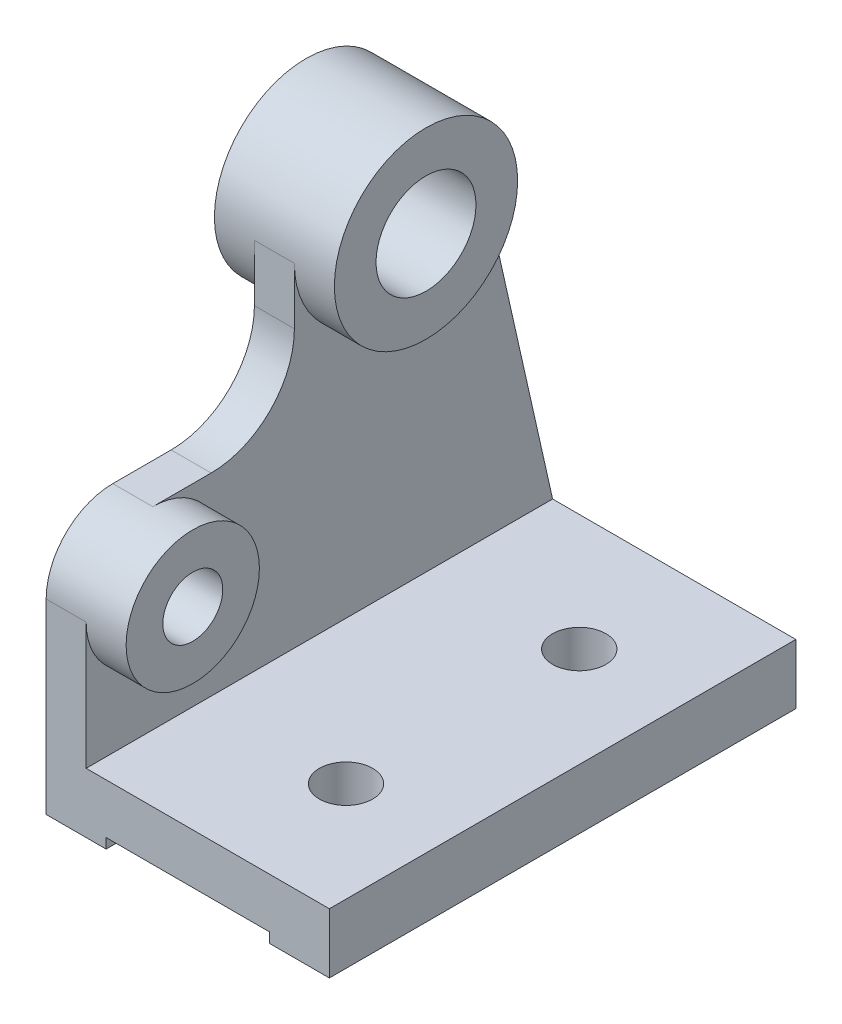
ISO-10303-21;
HEADER;
FILE_DESCRIPTION(('STEP AP214'),'2;1');
FILE_NAME('part.step','',(''),(''),'','','');
FILE_SCHEMA(('AUTOMOTIVE_DESIGN { 1 0 10303 214 1 1 1 1 }'));
ENDSEC;
DATA;
#1=APPLICATION_CONTEXT('core data for automotive mechanical design processes');
#2=APPLICATION_PROTOCOL_DEFINITION('international standard','automotive_design',2000,#1);
#3=PRODUCT_CONTEXT('',#1,'mechanical');
#4=PRODUCT('Part','Part','',(#3));
#5=PRODUCT_RELATED_PRODUCT_CATEGORY('part','',(#4));
#6=PRODUCT_DEFINITION_FORMATION('','',#4);
#7=PRODUCT_DEFINITION_CONTEXT('part definition',#1,'design');
#8=PRODUCT_DEFINITION('design','',#6,#7);
#9=PRODUCT_DEFINITION_SHAPE('','',#8);
#10=(LENGTH_UNIT() NAMED_UNIT(*) SI_UNIT(.MILLI.,.METRE.));
#11=(NAMED_UNIT(*) PLANE_ANGLE_UNIT() SI_UNIT($,.RADIAN.));
#12=(NAMED_UNIT(*) SI_UNIT($,.STERADIAN.) SOLID_ANGLE_UNIT());
#13=UNCERTAINTY_MEASURE_WITH_UNIT(LENGTH_MEASURE(1.E-05),#10,'distance_accuracy_value','');
#14=(GEOMETRIC_REPRESENTATION_CONTEXT(3) GLOBAL_UNCERTAINTY_ASSIGNED_CONTEXT((#13)) GLOBAL_UNIT_ASSIGNED_CONTEXT((#10,
#11,#12)) REPRESENTATION_CONTEXT('',''));
#15=CARTESIAN_POINT('',(0.,0.,0.));
#16=DIRECTION('',(0.,0.,1.));
#17=DIRECTION('',(1.,0.,0.));
#18=AXIS2_PLACEMENT_3D('',#15,#16,#17);
#19=CARTESIAN_POINT('',(-30.5,0.,0.));
#20=DIRECTION('',(-1.,0.,0.));
#21=DIRECTION('',(0.,0.,1.));
#22=AXIS2_PLACEMENT_3D('',#19,#20,#21);
#23=PLANE('',#22);
#24=CARTESIAN_POINT('',(-30.5,118.,-20.));
#25=DIRECTION('',(1.,0.,0.));
#26=DIRECTION('',(0.,0.,-1.));
#27=AXIS2_PLACEMENT_3D('',#24,#25,#26);
#28=CIRCLE('',#27,27.5);
#29=CARTESIAN_POINT('',(-30.5,118.,7.5));
#30=VERTEX_POINT('',#29);
#31=CARTESIAN_POINT('',(-30.5,118.,-47.5));
#32=VERTEX_POINT('',#31);
#33=EDGE_CURVE('E153',#30,#32,#28,.T.);
#34=ORIENTED_EDGE('',*,*,#33,.F.);
#35=DIRECTION('',(0.,-1.,0.));
#36=VECTOR('',#35,1.);
#37=CARTESIAN_POINT('',(-30.5,0.,7.49999999999995));
#38=LINE('',#37,#36);
#39=CARTESIAN_POINT('',(-30.5,101.,7.49999999999999));
#40=VERTEX_POINT('',#39);
#41=EDGE_CURVE('E160',#30,#40,#38,.T.);
#42=ORIENTED_EDGE('',*,*,#41,.T.);
#43=CARTESIAN_POINT('',(-30.5,101.,32.5));
#44=DIRECTION('',(-1.,0.,0.));
#45=DIRECTION('',(0.,0.,1.));
#46=AXIS2_PLACEMENT_3D('',#43,#44,#45);
#47=CIRCLE('',#46,25.);
#48=CARTESIAN_POINT('',(-30.5,76.,32.5));
#49=VERTEX_POINT('',#48);
#50=EDGE_CURVE('E178',#49,#40,#47,.F.);
#51=ORIENTED_EDGE('',*,*,#50,.F.);
#52=DIRECTION('',(0.,0.,-1.));
#53=VECTOR('',#52,1.);
#54=CARTESIAN_POINT('',(-30.5,76.,0.));
#55=LINE('',#54,#53);
#56=CARTESIAN_POINT('',(-30.5,76.,50.));
#57=VERTEX_POINT('',#56);
#58=EDGE_CURVE('E182',#57,#49,#55,.T.);
#59=ORIENTED_EDGE('',*,*,#58,.F.);
#60=CARTESIAN_POINT('',(-30.5,56.,50.));
#61=DIRECTION('',(-1.,0.,0.));
#62=DIRECTION('',(0.,0.,1.));
#63=AXIS2_PLACEMENT_3D('',#60,#61,#62);
#64=CIRCLE('',#63,20.);
#65=CARTESIAN_POINT('',(-30.5,56.,70.));
#66=VERTEX_POINT('',#65);
#67=EDGE_CURVE('E57',#66,#57,#64,.F.);
#68=ORIENTED_EDGE('',*,*,#67,.F.);
#69=DIRECTION('',(0.,1.,0.));
#70=VECTOR('',#69,1.);
#71=CARTESIAN_POINT('',(-30.5,0.,70.));
#72=LINE('',#71,#70);
#73=CARTESIAN_POINT('',(-30.5,18.,70.));
#74=VERTEX_POINT('',#73);
#75=EDGE_CURVE('E188',#74,#66,#72,.T.);
#76=ORIENTED_EDGE('',*,*,#75,.F.);
#77=DIRECTION('',(0.,0.,-1.));
#78=VECTOR('',#77,1.);
#79=CARTESIAN_POINT('',(-30.5,18.,0.));
#80=LINE('',#79,#78);
#81=CARTESIAN_POINT('',(-30.5,18.,-70.));
#82=VERTEX_POINT('',#81);
#83=EDGE_CURVE('E62',#74,#82,#80,.T.);
#84=ORIENTED_EDGE('',*,*,#83,.T.);
#85=DIRECTION('',(0.,0.975609756097561,0.219512195121951));
#86=VECTOR('',#85,1.);
#87=CARTESIAN_POINT('',(-30.5,15.8584176085663,-70.4818560380726));
#88=LINE('',#87,#86);
#89=EDGE_CURVE('E159',#82,#32,#88,.T.);
#90=ORIENTED_EDGE('',*,*,#89,.T.);
#91=EDGE_LOOP('',(#34,#42,#51,#59,#68,#76,#84,#90));
#92=FACE_BOUND('',#91,.T.);
#93=ADVANCED_FACE('F50',(#92),#23,.F.);
#94=CARTESIAN_POINT('',(0.,0.,0.));
#95=DIRECTION('',(0.,1.,0.));
#96=DIRECTION('',(0.,0.,1.));
#97=AXIS2_PLACEMENT_3D('',#94,#95,#96);
#98=PLANE('',#97);
#99=DIRECTION('',(-1.,0.,0.));
#100=VECTOR('',#99,1.);
#101=CARTESIAN_POINT('',(-42.5,0.,-70.));
#102=LINE('',#101,#100);
#103=CARTESIAN_POINT('',(-24.5,0.,-70.));
#104=VERTEX_POINT('',#103);
#105=CARTESIAN_POINT('',(-42.5,0.,-70.));
#106=VERTEX_POINT('',#105);
#107=EDGE_CURVE('E249',#104,#106,#102,.T.);
#108=ORIENTED_EDGE('',*,*,#107,.F.);
#109=DIRECTION('',(0.,0.,1.));
#110=VECTOR('',#109,1.);
#111=CARTESIAN_POINT('',(-24.5,0.,0.));
#112=LINE('',#111,#110);
#113=CARTESIAN_POINT('',(-24.5,0.,70.));
#114=VERTEX_POINT('',#113);
#115=EDGE_CURVE('E275',#104,#114,#112,.T.);
#116=ORIENTED_EDGE('',*,*,#115,.T.);
#117=DIRECTION('',(1.,0.,0.));
#118=VECTOR('',#117,1.);
#119=CARTESIAN_POINT('',(-42.5,0.,70.));
#120=LINE('',#119,#118);
#121=CARTESIAN_POINT('',(-42.5,0.,70.));
#122=VERTEX_POINT('',#121);
#123=EDGE_CURVE('E241',#122,#114,#120,.T.);
#124=ORIENTED_EDGE('',*,*,#123,.F.);
#125=DIRECTION('',(0.,0.,1.));
#126=VECTOR('',#125,1.);
#127=CARTESIAN_POINT('',(-42.5,0.,-70.));
#128=LINE('',#127,#126);
#129=EDGE_CURVE('E255',#106,#122,#128,.T.);
#130=ORIENTED_EDGE('',*,*,#129,.F.);
#131=EDGE_LOOP('',(#108,#116,#124,#130));
#132=FACE_BOUND('',#131,.T.);
#133=ADVANCED_FACE('F334',(#132),#98,.F.);
#134=CARTESIAN_POINT('',(42.5,18.,-70.));
#135=DIRECTION('',(-1.,0.,0.));
#136=DIRECTION('',(0.,0.,1.));
#137=AXIS2_PLACEMENT_3D('',#134,#135,#136);
#138=PLANE('',#137);
#139=DIRECTION('',(0.,0.,-1.));
#140=VECTOR('',#139,1.);
#141=CARTESIAN_POINT('',(42.5,0.,-70.));
#142=LINE('',#141,#140);
#143=CARTESIAN_POINT('',(42.5,0.,70.));
#144=VERTEX_POINT('',#143);
#145=CARTESIAN_POINT('',(42.5,0.,-70.));
#146=VERTEX_POINT('',#145);
#147=EDGE_CURVE('E236',#144,#146,#142,.T.);
#148=ORIENTED_EDGE('',*,*,#147,.T.);
#149=DIRECTION('',(0.,-1.,0.));
#150=VECTOR('',#149,1.);
#151=CARTESIAN_POINT('',(42.5,18.,-70.));
#152=LINE('',#151,#150);
#153=CARTESIAN_POINT('',(42.5,18.,-70.));
#154=VERTEX_POINT('',#153);
#155=EDGE_CURVE('E270',#154,#146,#152,.T.);
#156=ORIENTED_EDGE('',*,*,#155,.F.);
#157=DIRECTION('',(0.,0.,-1.));
#158=VECTOR('',#157,1.);
#159=CARTESIAN_POINT('',(42.5,18.,-70.));
#160=LINE('',#159,#158);
#161=CARTESIAN_POINT('',(42.5,18.,70.));
#162=VERTEX_POINT('',#161);
#163=EDGE_CURVE('E239',#162,#154,#160,.T.);
#164=ORIENTED_EDGE('',*,*,#163,.F.);
#165=DIRECTION('',(0.,-1.,0.));
#166=VECTOR('',#165,1.);
#167=CARTESIAN_POINT('',(42.5,18.,70.));
#168=LINE('',#167,#166);
#169=EDGE_CURVE('E250',#162,#144,#168,.T.);
#170=ORIENTED_EDGE('',*,*,#169,.T.);
#171=EDGE_LOOP('',(#148,#156,#164,#170));
#172=FACE_BOUND('',#171,.T.);
#173=ADVANCED_FACE('F47',(#172),#138,.F.);
#174=CARTESIAN_POINT('',(-42.5,18.,-70.));
#175=DIRECTION('',(0.,0.,1.));
#176=DIRECTION('',(1.,0.,0.));
#177=AXIS2_PLACEMENT_3D('',#174,#175,#176);
#178=PLANE('',#177);
#179=DIRECTION('',(-1.,0.,0.));
#180=VECTOR('',#179,1.);
#181=CARTESIAN_POINT('',(-42.5,3.,-70.));
#182=LINE('',#181,#180);
#183=CARTESIAN_POINT('',(24.5,3.,-70.));
#184=VERTEX_POINT('',#183);
#185=CARTESIAN_POINT('',(-24.5,3.,-70.));
#186=VERTEX_POINT('',#185);
#187=EDGE_CURVE('E234',#184,#186,#182,.T.);
#188=ORIENTED_EDGE('',*,*,#187,.T.);
#189=DIRECTION('',(0.,-1.,0.));
#190=VECTOR('',#189,1.);
#191=CARTESIAN_POINT('',(-24.5,18.,-70.));
#192=LINE('',#191,#190);
#193=EDGE_CURVE('E235',#186,#104,#192,.T.);
#194=ORIENTED_EDGE('',*,*,#193,.T.);
#195=ORIENTED_EDGE('',*,*,#107,.T.);
#196=DIRECTION('',(0.,-1.,0.));
#197=VECTOR('',#196,1.);
#198=CARTESIAN_POINT('',(-42.5,18.,-70.));
#199=LINE('',#198,#197);
#200=CARTESIAN_POINT('',(-42.5,18.,-70.));
#201=VERTEX_POINT('',#200);
#202=EDGE_CURVE('E262',#201,#106,#199,.T.);
#203=ORIENTED_EDGE('',*,*,#202,.F.);
#204=DIRECTION('',(-1.,0.,0.));
#205=VECTOR('',#204,1.);
#206=CARTESIAN_POINT('',(-30.5,18.,-70.));
#207=LINE('',#206,#205);
#208=EDGE_CURVE('E212',#82,#201,#207,.T.);
#209=ORIENTED_EDGE('',*,*,#208,.F.);
#210=DIRECTION('',(-1.,0.,0.));
#211=VECTOR('',#210,1.);
#212=CARTESIAN_POINT('',(-42.5,18.,-70.));
#213=LINE('',#212,#211);
#214=EDGE_CURVE('E245',#154,#82,#213,.T.);
#215=ORIENTED_EDGE('',*,*,#214,.F.);
#216=ORIENTED_EDGE('',*,*,#155,.T.);
#217=CARTESIAN_POINT('',(24.5,0.,-70.));
#218=VERTEX_POINT('',#217);
#219=EDGE_CURVE('E253',#146,#218,#102,.T.);
#220=ORIENTED_EDGE('',*,*,#219,.T.);
#221=DIRECTION('',(0.,1.,0.));
#222=VECTOR('',#221,1.);
#223=CARTESIAN_POINT('',(24.5,18.,-70.));
#224=LINE('',#223,#222);
#225=EDGE_CURVE('E75',#218,#184,#224,.T.);
#226=ORIENTED_EDGE('',*,*,#225,.T.);
#227=EDGE_LOOP('',(#188,#194,#195,#203,#209,#215,#216,#220,#226));
#228=FACE_BOUND('',#227,.T.);
#229=ADVANCED_FACE('F353',(#228),#178,.F.);
#230=CARTESIAN_POINT('',(-42.5,18.,-70.));
#231=DIRECTION('',(1.,0.,0.));
#232=DIRECTION('',(0.,0.,-1.));
#233=AXIS2_PLACEMENT_3D('',#230,#231,#232);
#234=PLANE('',#233);
#235=CARTESIAN_POINT('',(-42.5,118.,-20.));
#236=DIRECTION('',(-1.,0.,0.));
#237=DIRECTION('',(0.,0.,1.));
#238=AXIS2_PLACEMENT_3D('',#235,#236,#237);
#239=CIRCLE('',#238,27.5);
#240=CARTESIAN_POINT('',(-42.5,118.,-47.5));
#241=VERTEX_POINT('',#240);
#242=CARTESIAN_POINT('',(-42.5,118.,7.50000000000001));
#243=VERTEX_POINT('',#242);
#244=EDGE_CURVE('E11',#241,#243,#239,.T.);
#245=ORIENTED_EDGE('',*,*,#244,.F.);
#246=DIRECTION('',(0.,0.975609756097561,0.219512195121951));
#247=VECTOR('',#246,1.);
#248=CARTESIAN_POINT('',(-42.5,15.8584176085663,-70.4818560380726));
#249=LINE('',#248,#247);
#250=EDGE_CURVE('E200',#201,#241,#249,.T.);
#251=ORIENTED_EDGE('',*,*,#250,.F.);
#252=ORIENTED_EDGE('',*,*,#202,.T.);
#253=ORIENTED_EDGE('',*,*,#129,.T.);
#254=DIRECTION('',(0.,-1.,0.));
#255=VECTOR('',#254,1.);
#256=CARTESIAN_POINT('',(-42.5,18.,70.));
#257=LINE('',#256,#255);
#258=CARTESIAN_POINT('',(-42.5,56.,70.));
#259=VERTEX_POINT('',#258);
#260=EDGE_CURVE('E261',#259,#122,#257,.T.);
#261=ORIENTED_EDGE('',*,*,#260,.F.);
#262=CARTESIAN_POINT('',(-42.5,56.,50.));
#263=DIRECTION('',(-1.,0.,0.));
#264=DIRECTION('',(0.,0.,1.));
#265=AXIS2_PLACEMENT_3D('',#262,#263,#264);
#266=CIRCLE('',#265,20.);
#267=CARTESIAN_POINT('',(-42.5,76.,50.));
#268=VERTEX_POINT('',#267);
#269=EDGE_CURVE('E205',#259,#268,#266,.T.);
#270=ORIENTED_EDGE('',*,*,#269,.T.);
#271=DIRECTION('',(0.,0.,-1.));
#272=VECTOR('',#271,1.);
#273=CARTESIAN_POINT('',(-42.5,76.,0.));
#274=LINE('',#273,#272);
#275=CARTESIAN_POINT('',(-42.5,76.,32.5));
#276=VERTEX_POINT('',#275);
#277=EDGE_CURVE('E189',#268,#276,#274,.T.);
#278=ORIENTED_EDGE('',*,*,#277,.T.);
#279=CARTESIAN_POINT('',(-42.5,101.,32.5));
#280=DIRECTION('',(-1.,0.,0.));
#281=DIRECTION('',(0.,0.,1.));
#282=AXIS2_PLACEMENT_3D('',#279,#280,#281);
#283=CIRCLE('',#282,25.);
#284=CARTESIAN_POINT('',(-42.5,101.,7.49999999999999));
#285=VERTEX_POINT('',#284);
#286=EDGE_CURVE('E193',#276,#285,#283,.F.);
#287=ORIENTED_EDGE('',*,*,#286,.T.);
#288=DIRECTION('',(0.,-1.,0.));
#289=VECTOR('',#288,1.);
#290=CARTESIAN_POINT('',(-42.5,0.,7.49999999999995));
#291=LINE('',#290,#289);
#292=EDGE_CURVE('E197',#243,#285,#291,.T.);
#293=ORIENTED_EDGE('',*,*,#292,.F.);
#294=EDGE_LOOP('',(#245,#251,#252,#253,#261,#270,#278,#287,#293));
#295=FACE_BOUND('',#294,.T.);
#296=CARTESIAN_POINT('',(-42.5,56.,50.));
#297=DIRECTION('',(-1.,0.,0.));
#298=DIRECTION('',(0.,0.,1.));
#299=AXIS2_PLACEMENT_3D('',#296,#297,#298);
#300=CIRCLE('',#299,9.);
#301=CARTESIAN_POINT('',(-42.5,56.,59.));
#302=VERTEX_POINT('',#301);
#303=EDGE_CURVE('E202',#302,#302,#300,.T.);
#304=ORIENTED_EDGE('',*,*,#303,.F.);
#305=EDGE_LOOP('',(#304));
#306=FACE_BOUND('',#305,.T.);
#307=ADVANCED_FACE('F312',(#295,#306),#234,.F.);
#308=CARTESIAN_POINT('',(-42.5,18.,70.));
#309=DIRECTION('',(0.,0.,-1.));
#310=DIRECTION('',(-1.,0.,0.));
#311=AXIS2_PLACEMENT_3D('',#308,#309,#310);
#312=PLANE('',#311);
#313=ORIENTED_EDGE('',*,*,#123,.T.);
#314=DIRECTION('',(0.,-1.,0.));
#315=VECTOR('',#314,1.);
#316=CARTESIAN_POINT('',(-24.5,0.,70.));
#317=LINE('',#316,#315);
#318=CARTESIAN_POINT('',(-24.5,3.,70.));
#319=VERTEX_POINT('',#318);
#320=EDGE_CURVE('E223',#319,#114,#317,.T.);
#321=ORIENTED_EDGE('',*,*,#320,.F.);
#322=DIRECTION('',(-1.,0.,0.));
#323=VECTOR('',#322,1.);
#324=CARTESIAN_POINT('',(-24.5,3.,70.));
#325=LINE('',#324,#323);
#326=CARTESIAN_POINT('',(24.5,3.,70.));
#327=VERTEX_POINT('',#326);
#328=EDGE_CURVE('E225',#327,#319,#325,.T.);
#329=ORIENTED_EDGE('',*,*,#328,.F.);
#330=DIRECTION('',(0.,1.,0.));
#331=VECTOR('',#330,1.);
#332=CARTESIAN_POINT('',(24.5,0.,70.));
#333=LINE('',#332,#331);
#334=CARTESIAN_POINT('',(24.5,0.,70.));
#335=VERTEX_POINT('',#334);
#336=EDGE_CURVE('E209',#335,#327,#333,.T.);
#337=ORIENTED_EDGE('',*,*,#336,.F.);
#338=EDGE_CURVE('E258',#335,#144,#120,.T.);
#339=ORIENTED_EDGE('',*,*,#338,.T.);
#340=ORIENTED_EDGE('',*,*,#169,.F.);
#341=DIRECTION('',(1.,0.,0.));
#342=VECTOR('',#341,1.);
#343=CARTESIAN_POINT('',(-42.5,18.,70.));
#344=LINE('',#343,#342);
#345=EDGE_CURVE('E244',#74,#162,#344,.T.);
#346=ORIENTED_EDGE('',*,*,#345,.F.);
#347=ORIENTED_EDGE('',*,*,#75,.T.);
#348=DIRECTION('',(-1.,0.,0.));
#349=VECTOR('',#348,1.);
#350=CARTESIAN_POINT('',(-30.5,56.,70.));
#351=LINE('',#350,#349);
#352=EDGE_CURVE('E211',#66,#259,#351,.T.);
#353=ORIENTED_EDGE('',*,*,#352,.T.);
#354=ORIENTED_EDGE('',*,*,#260,.T.);
#355=EDGE_LOOP('',(#313,#321,#329,#337,#339,#340,#346,#347,#353,#354));
#356=FACE_BOUND('',#355,.T.);
#357=ADVANCED_FACE('F325',(#356),#312,.F.);
#358=CARTESIAN_POINT('',(0.,18.,0.));
#359=DIRECTION('',(0.,1.,0.));
#360=DIRECTION('',(0.,0.,1.));
#361=AXIS2_PLACEMENT_3D('',#358,#359,#360);
#362=PLANE('',#361);
#363=CARTESIAN_POINT('',(12.5,18.,-35.));
#364=DIRECTION('',(0.,1.,0.));
#365=DIRECTION('',(0.,0.,1.));
#366=AXIS2_PLACEMENT_3D('',#363,#364,#365);
#367=CIRCLE('',#366,8.);
#368=CARTESIAN_POINT('',(12.5,18.,-27.));
#369=VERTEX_POINT('',#368);
#370=EDGE_CURVE('E280',#369,#369,#367,.T.);
#371=ORIENTED_EDGE('',*,*,#370,.F.);
#372=EDGE_LOOP('',(#371));
#373=FACE_BOUND('',#372,.T.);
#374=CARTESIAN_POINT('',(12.5,18.,35.));
#375=DIRECTION('',(0.,1.,0.));
#376=DIRECTION('',(0.,0.,1.));
#377=AXIS2_PLACEMENT_3D('',#374,#375,#376);
#378=CIRCLE('',#377,8.);
#379=CARTESIAN_POINT('',(12.5,18.,43.));
#380=VERTEX_POINT('',#379);
#381=EDGE_CURVE('E285',#380,#380,#378,.T.);
#382=ORIENTED_EDGE('',*,*,#381,.F.);
#383=EDGE_LOOP('',(#382));
#384=FACE_BOUND('',#383,.T.);
#385=ORIENTED_EDGE('',*,*,#83,.F.);
#386=ORIENTED_EDGE('',*,*,#345,.T.);
#387=ORIENTED_EDGE('',*,*,#163,.T.);
#388=ORIENTED_EDGE('',*,*,#214,.T.);
#389=EDGE_LOOP('',(#385,#386,#387,#388));
#390=FACE_BOUND('',#389,.T.);
#391=ADVANCED_FACE('F348',(#373,#384,#390),#362,.T.);
#392=ORIENTED_EDGE('',*,*,#338,.F.);
#393=DIRECTION('',(0.,0.,-1.));
#394=VECTOR('',#393,1.);
#395=CARTESIAN_POINT('',(24.5,0.,0.));
#396=LINE('',#395,#394);
#397=EDGE_CURVE('E269',#335,#218,#396,.T.);
#398=ORIENTED_EDGE('',*,*,#397,.T.);
#399=ORIENTED_EDGE('',*,*,#219,.F.);
#400=ORIENTED_EDGE('',*,*,#147,.F.);
#401=EDGE_LOOP('',(#392,#398,#399,#400));
#402=FACE_BOUND('',#401,.T.);
#403=ADVANCED_FACE('F347',(#402),#98,.F.);
#404=CARTESIAN_POINT('',(-24.5,3.,-80.));
#405=DIRECTION('',(0.,1.,0.));
#406=DIRECTION('',(0.,0.,1.));
#407=AXIS2_PLACEMENT_3D('',#404,#405,#406);
#408=PLANE('',#407);
#409=CARTESIAN_POINT('',(12.5,3.,-35.));
#410=DIRECTION('',(0.,1.,0.));
#411=DIRECTION('',(0.,0.,1.));
#412=AXIS2_PLACEMENT_3D('',#409,#410,#411);
#413=CIRCLE('',#412,8.);
#414=CARTESIAN_POINT('',(12.5,3.,-27.));
#415=VERTEX_POINT('',#414);
#416=EDGE_CURVE('E51',#415,#415,#413,.T.);
#417=ORIENTED_EDGE('',*,*,#416,.T.);
#418=EDGE_LOOP('',(#417));
#419=FACE_BOUND('',#418,.T.);
#420=CARTESIAN_POINT('',(12.5,3.,35.));
#421=DIRECTION('',(0.,1.,0.));
#422=DIRECTION('',(0.,0.,1.));
#423=AXIS2_PLACEMENT_3D('',#420,#421,#422);
#424=CIRCLE('',#423,8.);
#425=CARTESIAN_POINT('',(12.5,3.,43.));
#426=VERTEX_POINT('',#425);
#427=EDGE_CURVE('E274',#426,#426,#424,.T.);
#428=ORIENTED_EDGE('',*,*,#427,.T.);
#429=EDGE_LOOP('',(#428));
#430=FACE_BOUND('',#429,.T.);
#431=DIRECTION('',(0.,0.,1.));
#432=VECTOR('',#431,1.);
#433=CARTESIAN_POINT('',(24.5,3.,-80.));
#434=LINE('',#433,#432);
#435=EDGE_CURVE('E230',#184,#327,#434,.T.);
#436=ORIENTED_EDGE('',*,*,#435,.T.);
#437=ORIENTED_EDGE('',*,*,#328,.T.);
#438=DIRECTION('',(0.,0.,1.));
#439=VECTOR('',#438,1.);
#440=CARTESIAN_POINT('',(-24.5,3.,-80.));
#441=LINE('',#440,#439);
#442=EDGE_CURVE('E226',#186,#319,#441,.T.);
#443=ORIENTED_EDGE('',*,*,#442,.F.);
#444=ORIENTED_EDGE('',*,*,#187,.F.);
#445=EDGE_LOOP('',(#436,#437,#443,#444));
#446=FACE_BOUND('',#445,.T.);
#447=ADVANCED_FACE('F341',(#419,#430,#446),#408,.F.);
#448=CARTESIAN_POINT('',(-24.5,0.,-80.));
#449=DIRECTION('',(-1.,0.,0.));
#450=DIRECTION('',(0.,0.,1.));
#451=AXIS2_PLACEMENT_3D('',#448,#449,#450);
#452=PLANE('',#451);
#453=ORIENTED_EDGE('',*,*,#442,.T.);
#454=ORIENTED_EDGE('',*,*,#320,.T.);
#455=ORIENTED_EDGE('',*,*,#115,.F.);
#456=ORIENTED_EDGE('',*,*,#193,.F.);
#457=EDGE_LOOP('',(#453,#454,#455,#456));
#458=FACE_BOUND('',#457,.T.);
#459=ADVANCED_FACE('F336',(#458),#452,.F.);
#460=CARTESIAN_POINT('',(24.5,0.,-80.));
#461=DIRECTION('',(1.,0.,0.));
#462=DIRECTION('',(0.,0.,-1.));
#463=AXIS2_PLACEMENT_3D('',#460,#461,#462);
#464=PLANE('',#463);
#465=ORIENTED_EDGE('',*,*,#397,.F.);
#466=ORIENTED_EDGE('',*,*,#336,.T.);
#467=ORIENTED_EDGE('',*,*,#435,.F.);
#468=ORIENTED_EDGE('',*,*,#225,.F.);
#469=EDGE_LOOP('',(#465,#466,#467,#468));
#470=FACE_BOUND('',#469,.T.);
#471=ADVANCED_FACE('F345',(#470),#464,.F.);
#472=CARTESIAN_POINT('',(-30.5,76.,0.));
#473=DIRECTION('',(0.,1.,0.));
#474=DIRECTION('',(0.,0.,1.));
#475=AXIS2_PLACEMENT_3D('',#472,#473,#474);
#476=PLANE('',#475);
#477=ORIENTED_EDGE('',*,*,#277,.F.);
#478=DIRECTION('',(-1.,0.,0.));
#479=VECTOR('',#478,1.);
#480=CARTESIAN_POINT('',(-30.5,76.,50.));
#481=LINE('',#480,#479);
#482=EDGE_CURVE('E208',#57,#268,#481,.T.);
#483=ORIENTED_EDGE('',*,*,#482,.F.);
#484=ORIENTED_EDGE('',*,*,#58,.T.);
#485=DIRECTION('',(-1.,0.,0.));
#486=VECTOR('',#485,1.);
#487=CARTESIAN_POINT('',(-30.5,76.,32.5));
#488=LINE('',#487,#486);
#489=EDGE_CURVE('E187',#49,#276,#488,.T.);
#490=ORIENTED_EDGE('',*,*,#489,.T.);
#491=EDGE_LOOP('',(#477,#483,#484,#490));
#492=FACE_BOUND('',#491,.T.);
#493=ADVANCED_FACE('F306',(#492),#476,.T.);
#494=CARTESIAN_POINT('',(-30.5,56.,50.));
#495=DIRECTION('',(-1.,0.,0.));
#496=DIRECTION('',(0.,0.,1.));
#497=AXIS2_PLACEMENT_3D('',#494,#495,#496);
#498=CYLINDRICAL_SURFACE('',#497,20.);
#499=ORIENTED_EDGE('',*,*,#269,.F.);
#500=ORIENTED_EDGE('',*,*,#352,.F.);
#501=ORIENTED_EDGE('',*,*,#67,.T.);
#502=ORIENTED_EDGE('',*,*,#482,.T.);
#503=EDGE_LOOP('',(#499,#500,#501,#502));
#504=FACE_BOUND('',#503,.T.);
#505=CARTESIAN_POINT('',(-18.5,56.,50.));
#506=DIRECTION('',(1.,0.,0.));
#507=DIRECTION('',(0.,0.,-1.));
#508=AXIS2_PLACEMENT_3D('',#505,#506,#507);
#509=CIRCLE('',#508,20.);
#510=CARTESIAN_POINT('',(-18.5,56.,30.));
#511=VERTEX_POINT('',#510);
#512=EDGE_CURVE('E192',#511,#511,#509,.T.);
#513=ORIENTED_EDGE('',*,*,#512,.F.);
#514=EDGE_LOOP('',(#513));
#515=FACE_BOUND('',#514,.T.);
#516=ADVANCED_FACE('F317',(#504,#515),#498,.T.);
#517=CARTESIAN_POINT('',(-30.5,15.8584176085663,-70.4818560380726));
#518=DIRECTION('',(0.,-0.219512195121951,0.975609756097561));
#519=DIRECTION('',(0.,-0.975609756097561,-0.219512195121951));
#520=AXIS2_PLACEMENT_3D('',#517,#518,#519);
#521=PLANE('',#520);
#522=ORIENTED_EDGE('',*,*,#250,.T.);
#523=DIRECTION('',(-1.,0.,0.));
#524=VECTOR('',#523,1.);
#525=CARTESIAN_POINT('',(-30.5,118.,-47.5));
#526=LINE('',#525,#524);
#527=EDGE_CURVE('E171',#32,#241,#526,.T.);
#528=ORIENTED_EDGE('',*,*,#527,.F.);
#529=ORIENTED_EDGE('',*,*,#89,.F.);
#530=ORIENTED_EDGE('',*,*,#208,.T.);
#531=EDGE_LOOP('',(#522,#528,#529,#530));
#532=FACE_BOUND('',#531,.T.);
#533=ADVANCED_FACE('F324',(#532),#521,.F.);
#534=CARTESIAN_POINT('',(-30.5,118.,-20.));
#535=DIRECTION('',(-1.,0.,0.));
#536=DIRECTION('',(0.,0.,1.));
#537=AXIS2_PLACEMENT_3D('',#534,#535,#536);
#538=CYLINDRICAL_SURFACE('',#537,27.5);
#539=ORIENTED_EDGE('',*,*,#527,.T.);
#540=ORIENTED_EDGE('',*,*,#244,.T.);
#541=DIRECTION('',(-1.,0.,0.));
#542=VECTOR('',#541,1.);
#543=CARTESIAN_POINT('',(-30.5,118.,7.5));
#544=LINE('',#543,#542);
#545=EDGE_CURVE('E169',#30,#243,#544,.T.);
#546=ORIENTED_EDGE('',*,*,#545,.F.);
#547=ORIENTED_EDGE('',*,*,#33,.T.);
#548=EDGE_LOOP('',(#539,#540,#546,#547));
#549=FACE_BOUND('',#548,.T.);
#550=CARTESIAN_POINT('',(-54.5,118.,-20.));
#551=DIRECTION('',(-1.,0.,0.));
#552=DIRECTION('',(0.,0.,1.));
#553=AXIS2_PLACEMENT_3D('',#550,#551,#552);
#554=CIRCLE('',#553,27.5);
#555=CARTESIAN_POINT('',(-54.5,118.,7.50000000000001));
#556=VERTEX_POINT('',#555);
#557=EDGE_CURVE('E298',#556,#556,#554,.T.);
#558=ORIENTED_EDGE('',*,*,#557,.F.);
#559=EDGE_LOOP('',(#558));
#560=FACE_BOUND('',#559,.T.);
#561=CARTESIAN_POINT('',(-18.5,118.,-20.));
#562=DIRECTION('',(1.,0.,0.));
#563=DIRECTION('',(0.,0.,-1.));
#564=AXIS2_PLACEMENT_3D('',#561,#562,#563);
#565=CIRCLE('',#564,27.5);
#566=CARTESIAN_POINT('',(-18.5,118.,-47.5));
#567=VERTEX_POINT('',#566);
#568=EDGE_CURVE('E163',#567,#567,#565,.T.);
#569=ORIENTED_EDGE('',*,*,#568,.F.);
#570=EDGE_LOOP('',(#569));
#571=FACE_BOUND('',#570,.T.);
#572=ADVANCED_FACE('F166',(#549,#560,#571),#538,.T.);
#573=CARTESIAN_POINT('',(-30.5,0.,7.49999999999995));
#574=DIRECTION('',(0.,0.,-1.));
#575=DIRECTION('',(0.,1.,0.));
#576=AXIS2_PLACEMENT_3D('',#573,#574,#575);
#577=PLANE('',#576);
#578=ORIENTED_EDGE('',*,*,#292,.T.);
#579=DIRECTION('',(-1.,0.,0.));
#580=VECTOR('',#579,1.);
#581=CARTESIAN_POINT('',(-30.5,101.,7.49999999999999));
#582=LINE('',#581,#580);
#583=EDGE_CURVE('E172',#40,#285,#582,.T.);
#584=ORIENTED_EDGE('',*,*,#583,.F.);
#585=ORIENTED_EDGE('',*,*,#41,.F.);
#586=ORIENTED_EDGE('',*,*,#545,.T.);
#587=EDGE_LOOP('',(#578,#584,#585,#586));
#588=FACE_BOUND('',#587,.T.);
#589=ADVANCED_FACE('F176',(#588),#577,.F.);
#590=CARTESIAN_POINT('',(-30.5,56.,50.));
#591=DIRECTION('',(-1.,0.,0.));
#592=DIRECTION('',(0.,0.,1.));
#593=AXIS2_PLACEMENT_3D('',#590,#591,#592);
#594=CYLINDRICAL_SURFACE('',#593,9.);
#595=ORIENTED_EDGE('',*,*,#303,.T.);
#596=EDGE_LOOP('',(#595));
#597=FACE_BOUND('',#596,.T.);
#598=CARTESIAN_POINT('',(-18.5,56.,50.));
#599=DIRECTION('',(1.,0.,0.));
#600=DIRECTION('',(0.,0.,-1.));
#601=AXIS2_PLACEMENT_3D('',#598,#599,#600);
#602=CIRCLE('',#601,9.);
#603=CARTESIAN_POINT('',(-18.5,56.,41.));
#604=VERTEX_POINT('',#603);
#605=EDGE_CURVE('E296',#604,#604,#602,.T.);
#606=ORIENTED_EDGE('',*,*,#605,.T.);
#607=EDGE_LOOP('',(#606));
#608=FACE_BOUND('',#607,.T.);
#609=ADVANCED_FACE('F376',(#597,#608),#594,.F.);
#610=CARTESIAN_POINT('',(-30.5,101.,32.5));
#611=DIRECTION('',(-1.,0.,0.));
#612=DIRECTION('',(0.,0.,1.));
#613=AXIS2_PLACEMENT_3D('',#610,#611,#612);
#614=CYLINDRICAL_SURFACE('',#613,25.);
#615=ORIENTED_EDGE('',*,*,#286,.F.);
#616=ORIENTED_EDGE('',*,*,#489,.F.);
#617=ORIENTED_EDGE('',*,*,#50,.T.);
#618=ORIENTED_EDGE('',*,*,#583,.T.);
#619=EDGE_LOOP('',(#615,#616,#617,#618));
#620=FACE_BOUND('',#619,.T.);
#621=ADVANCED_FACE('F311',(#620),#614,.F.);
#622=CARTESIAN_POINT('',(-30.5,118.,-20.));
#623=DIRECTION('',(-1.,0.,0.));
#624=DIRECTION('',(0.,0.,1.));
#625=AXIS2_PLACEMENT_3D('',#622,#623,#624);
#626=CYLINDRICAL_SURFACE('',#625,15.);
#627=CARTESIAN_POINT('',(-54.5,118.,-20.));
#628=DIRECTION('',(-1.,0.,0.));
#629=DIRECTION('',(0.,0.,1.));
#630=AXIS2_PLACEMENT_3D('',#627,#628,#629);
#631=CIRCLE('',#630,15.);
#632=CARTESIAN_POINT('',(-54.5,118.,-5.00000000000002));
#633=VERTEX_POINT('',#632);
#634=EDGE_CURVE('E295',#633,#633,#631,.T.);
#635=ORIENTED_EDGE('',*,*,#634,.T.);
#636=EDGE_LOOP('',(#635));
#637=FACE_BOUND('',#636,.T.);
#638=CARTESIAN_POINT('',(-18.5,118.,-20.));
#639=DIRECTION('',(1.,0.,0.));
#640=DIRECTION('',(0.,0.,-1.));
#641=AXIS2_PLACEMENT_3D('',#638,#639,#640);
#642=CIRCLE('',#641,15.);
#643=CARTESIAN_POINT('',(-18.5,118.,-35.));
#644=VERTEX_POINT('',#643);
#645=EDGE_CURVE('E164',#644,#644,#642,.T.);
#646=ORIENTED_EDGE('',*,*,#645,.T.);
#647=EDGE_LOOP('',(#646));
#648=FACE_BOUND('',#647,.T.);
#649=ADVANCED_FACE('F375',(#637,#648),#626,.F.);
#650=CARTESIAN_POINT('',(-18.5,56.,50.));
#651=DIRECTION('',(1.,0.,0.));
#652=DIRECTION('',(0.,0.,-1.));
#653=AXIS2_PLACEMENT_3D('',#650,#651,#652);
#654=PLANE('',#653);
#655=ORIENTED_EDGE('',*,*,#512,.T.);
#656=EDGE_LOOP('',(#655));
#657=FACE_BOUND('',#656,.T.);
#658=ORIENTED_EDGE('',*,*,#605,.F.);
#659=EDGE_LOOP('',(#658));
#660=FACE_BOUND('',#659,.T.);
#661=ADVANCED_FACE('F367',(#657,#660),#654,.T.);
#662=CARTESIAN_POINT('',(-54.5,118.,-20.));
#663=DIRECTION('',(-1.,0.,0.));
#664=DIRECTION('',(0.,0.,1.));
#665=AXIS2_PLACEMENT_3D('',#662,#663,#664);
#666=PLANE('',#665);
#667=ORIENTED_EDGE('',*,*,#557,.T.);
#668=EDGE_LOOP('',(#667));
#669=FACE_BOUND('',#668,.T.);
#670=ORIENTED_EDGE('',*,*,#634,.F.);
#671=EDGE_LOOP('',(#670));
#672=FACE_BOUND('',#671,.T.);
#673=ADVANCED_FACE('F433',(#669,#672),#666,.T.);
#674=CARTESIAN_POINT('',(-18.5,118.,-20.));
#675=DIRECTION('',(1.,0.,0.));
#676=DIRECTION('',(0.,0.,-1.));
#677=AXIS2_PLACEMENT_3D('',#674,#675,#676);
#678=PLANE('',#677);
#679=ORIENTED_EDGE('',*,*,#568,.T.);
#680=EDGE_LOOP('',(#679));
#681=FACE_BOUND('',#680,.T.);
#682=ORIENTED_EDGE('',*,*,#645,.F.);
#683=EDGE_LOOP('',(#682));
#684=FACE_BOUND('',#683,.T.);
#685=ADVANCED_FACE('F443',(#681,#684),#678,.T.);
#686=CARTESIAN_POINT('',(12.5,-2.,35.));
#687=DIRECTION('',(0.,1.,0.));
#688=DIRECTION('',(0.,0.,1.));
#689=AXIS2_PLACEMENT_3D('',#686,#687,#688);
#690=CYLINDRICAL_SURFACE('',#689,8.);
#691=ORIENTED_EDGE('',*,*,#381,.T.);
#692=EDGE_LOOP('',(#691));
#693=FACE_BOUND('',#692,.T.);
#694=ORIENTED_EDGE('',*,*,#427,.F.);
#695=EDGE_LOOP('',(#694));
#696=FACE_BOUND('',#695,.T.);
#697=ADVANCED_FACE('F485',(#693,#696),#690,.F.);
#698=CARTESIAN_POINT('',(12.5,-2.,-35.));
#699=DIRECTION('',(0.,1.,0.));
#700=DIRECTION('',(0.,0.,1.));
#701=AXIS2_PLACEMENT_3D('',#698,#699,#700);
#702=CYLINDRICAL_SURFACE('',#701,8.);
#703=ORIENTED_EDGE('',*,*,#370,.T.);
#704=EDGE_LOOP('',(#703));
#705=FACE_BOUND('',#704,.T.);
#706=ORIENTED_EDGE('',*,*,#416,.F.);
#707=EDGE_LOOP('',(#706));
#708=FACE_BOUND('',#707,.T.);
#709=ADVANCED_FACE('F492',(#705,#708),#702,.F.);
#710=CLOSED_SHELL('',(#93,#133,#173,#229,#307,#357,#391,#403,#447,#459,#471,#493,#516,#533,#572,
#589,#609,#621,#649,#661,#673,#685,#697,#709));
#711=MANIFOLD_SOLID_BREP('B2',#710);
#712=ADVANCED_BREP_SHAPE_REPRESENTATION('',(#18,#711),#14);
#713=SHAPE_DEFINITION_REPRESENTATION(#9,#712);
ENDSEC;
END-ISO-10303-21;
